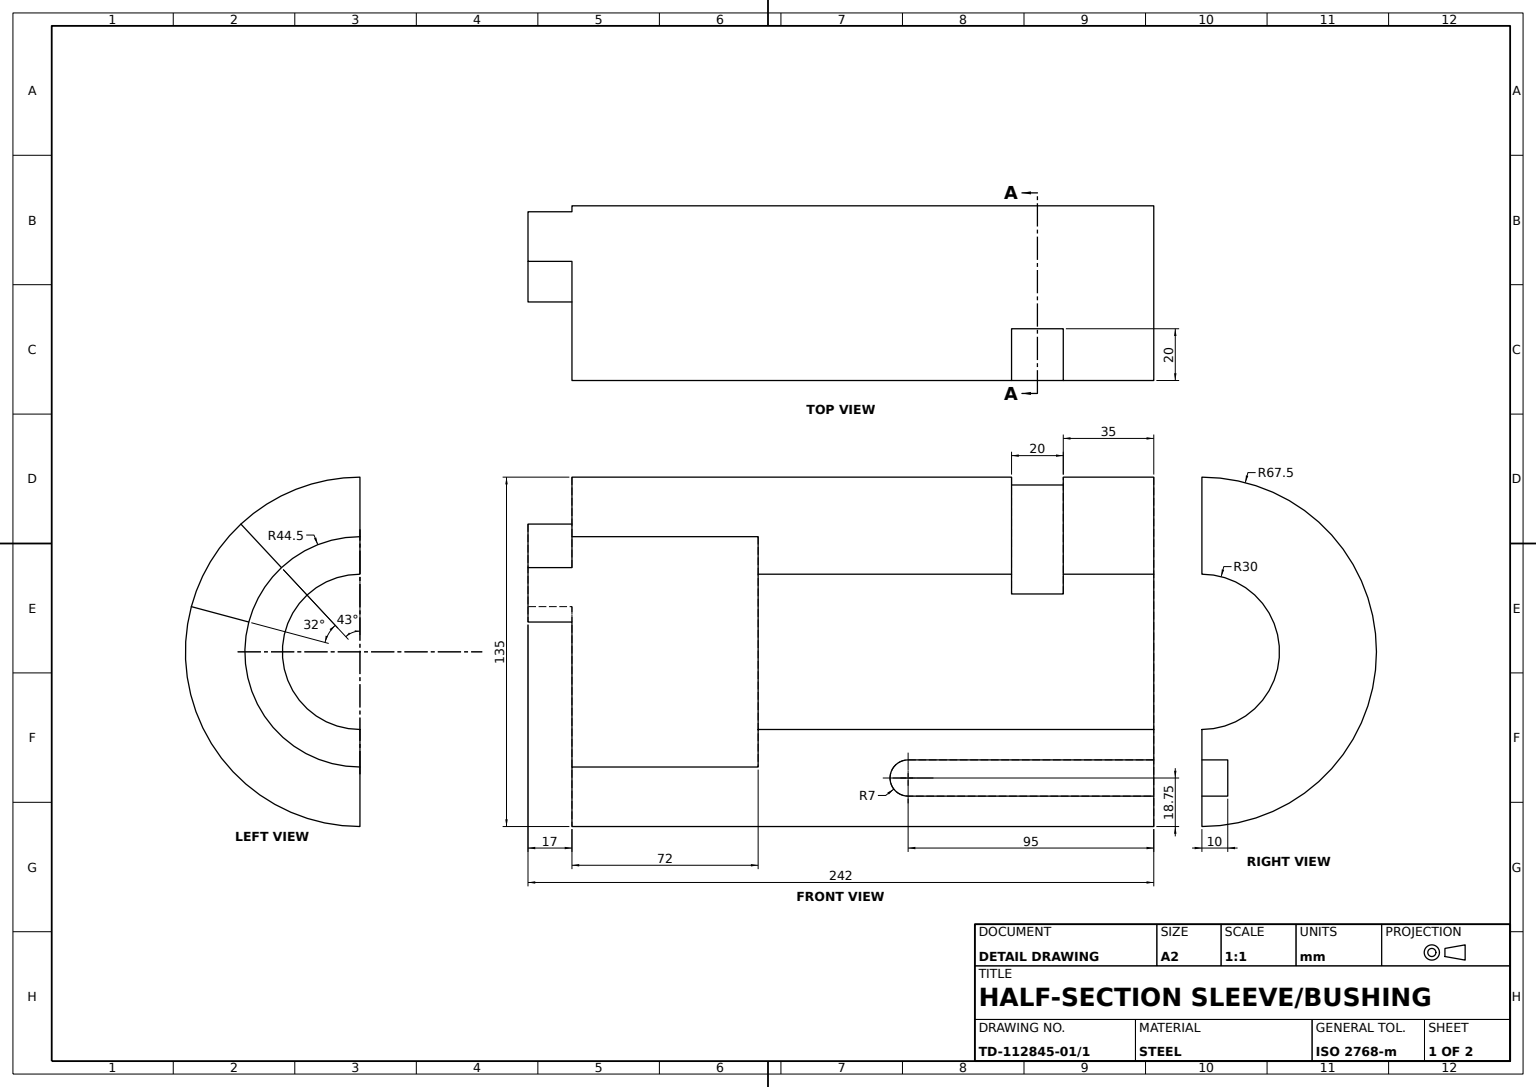
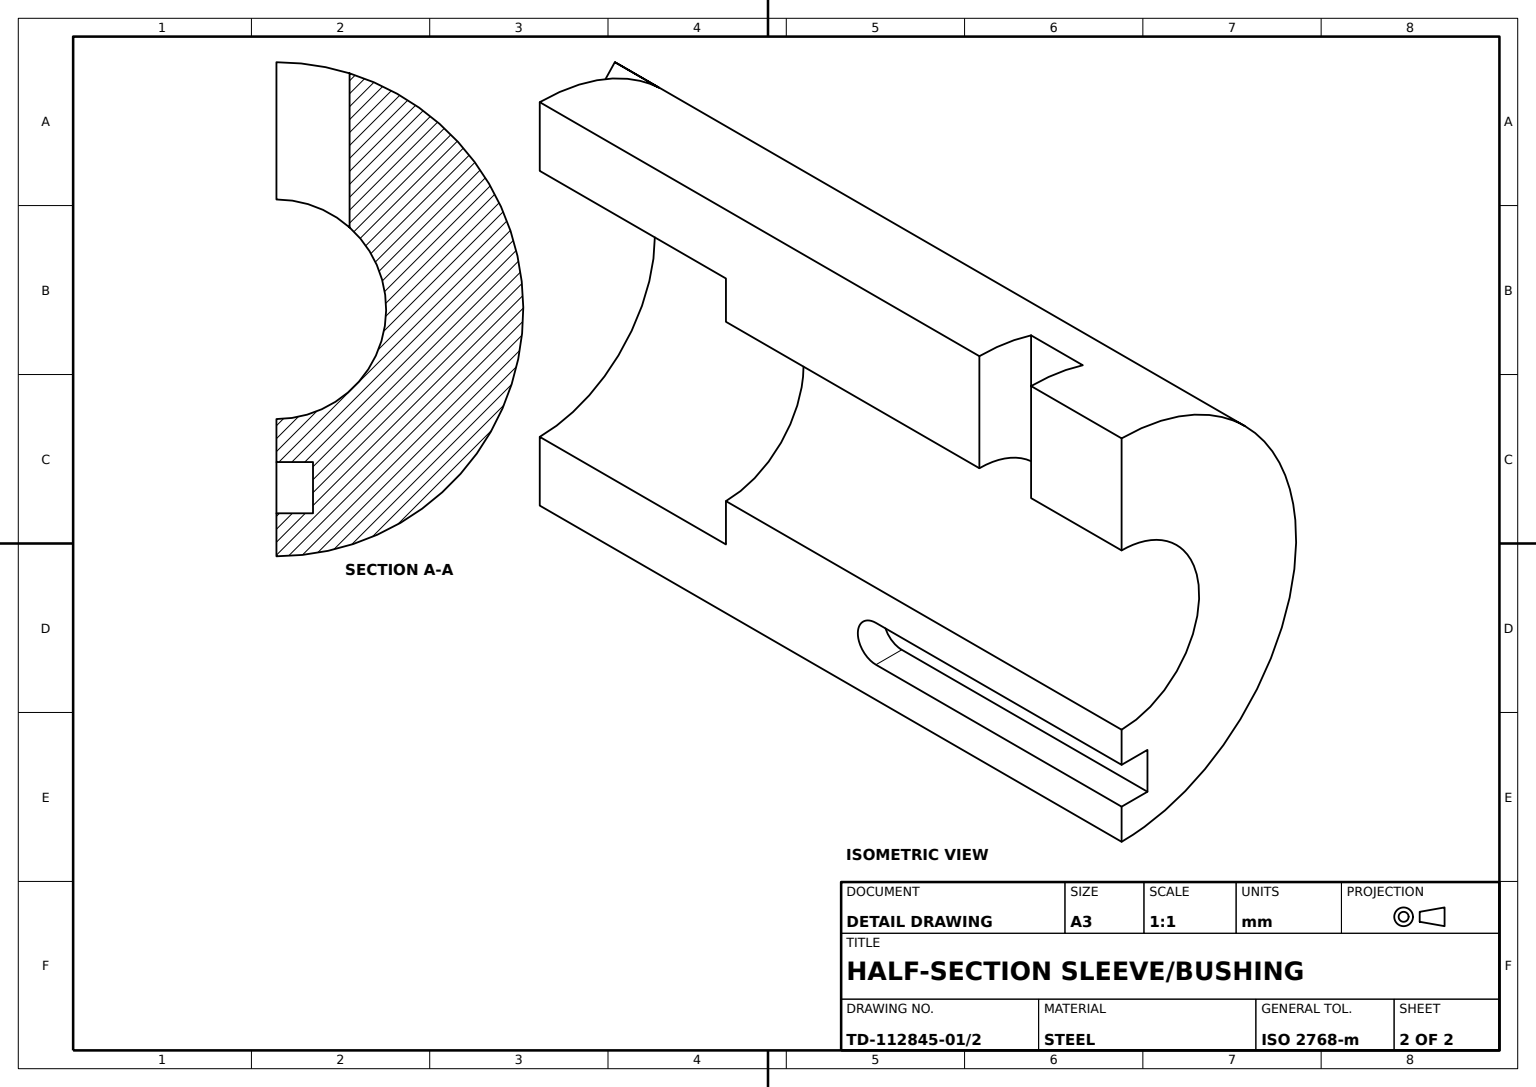
from build123d import *

# Parameters (mm, degrees)
BASE_BLOCK_60X135X225_DEPTH = 225
BORE_PROFILE_SKETCH_W       = 72
BORE_PROFILE_SKETCH_H       = 44.5
SECTOR_START                = 17
SECTOR_BOSS_32DEG_X17_DEPTH = 17
END_NOTCH_SKETCH_W          = 20
END_NOTCH_SKETCH_H          = 20
END_NOTCH_20X35_DEPTH       = 97
SLOT_7X95_DEPTH             = 10


with BuildPart() as part:
    # Base Block Sketch → Base Block 60x135x225 (new body)
    with BuildSketch(Plane.XY):
        with BuildLine():
            Line((0, 67.5), (0, 30))
            ThreePointArc((0, 30), (-30, 0), (0, -30))
            Line((0, -30), (0, -67.5))
            ThreePointArc((0, -67.5), (-67.5, 0), (0, 67.5))
        make_face()
    extrude(amount=-BASE_BLOCK_60X135X225_DEPTH)

    # Bore Profile Sketch → Bore Revolve Cut (revolve, cut)
    with BuildSketch(Plane(origin=(0, 0, 0), x_dir=(0, 0, -1), z_dir=(1, 0, 0))):
        with Locations((36, 22.25)):
            Rectangle(BORE_PROFILE_SKETCH_W, BORE_PROFILE_SKETCH_H)
    revolve(axis=Axis((0, 0, 32.736961991), (0, 0, -1)), mode=Mode.SUBTRACT)

    # Sector Boss Sketch → Sector Boss 32deg x17 (add)
    with BuildSketch(Plane.XY.offset(SECTOR_START)):
        with BuildLine():
            Line((-30.348927023, 32.545239722), (-46.034889304, 49.366374859))
            ThreePointArc((-46.034889304, 49.366374859), (-57.858792797, 34.765070056), (-65.199993275, 17.470285544))
            Line((-65.199993275, 17.470285544), (-42.98369927, 11.517447507))
            ThreePointArc((-42.98369927, 11.517447507), (-38.143944881, 22.919194333), (-30.348927023, 32.545239722))
        make_face()
    extrude(amount=-SECTOR_BOSS_32DEG_X17_DEPTH)

    # End Notch Sketch → End Notch 20x35 (cut)
    with BuildSketch(Plane(origin=(0, 0, 0), x_dir=(1, 0, 0), z_dir=(0, 1, 0))):
        with Locations((-10, 180)):
            Rectangle(END_NOTCH_SKETCH_W, END_NOTCH_SKETCH_H)
    extrude(amount=END_NOTCH_20X35_DEPTH, mode=Mode.SUBTRACT)

    # Slot Sketch → Slot 7x95 (cut)
    with BuildSketch(Plane(origin=(0, 0, 0), x_dir=(0, 0, -1), z_dir=(1, 0, 0))):
        with BuildLine():
            Line((239.283215377, -55.75), (130, -55.75))
            ThreePointArc((130, -55.75), (123, -48.75), (130, -41.75))
            Line((130, -41.75), (239.283215377, -41.75))
            ThreePointArc((239.283215377, -41.75), (246.283215377, -48.75), (239.283215377, -55.75))
        make_face()
    extrude(amount=-SLOT_7X95_DEPTH, mode=Mode.SUBTRACT)


solid = part.part
